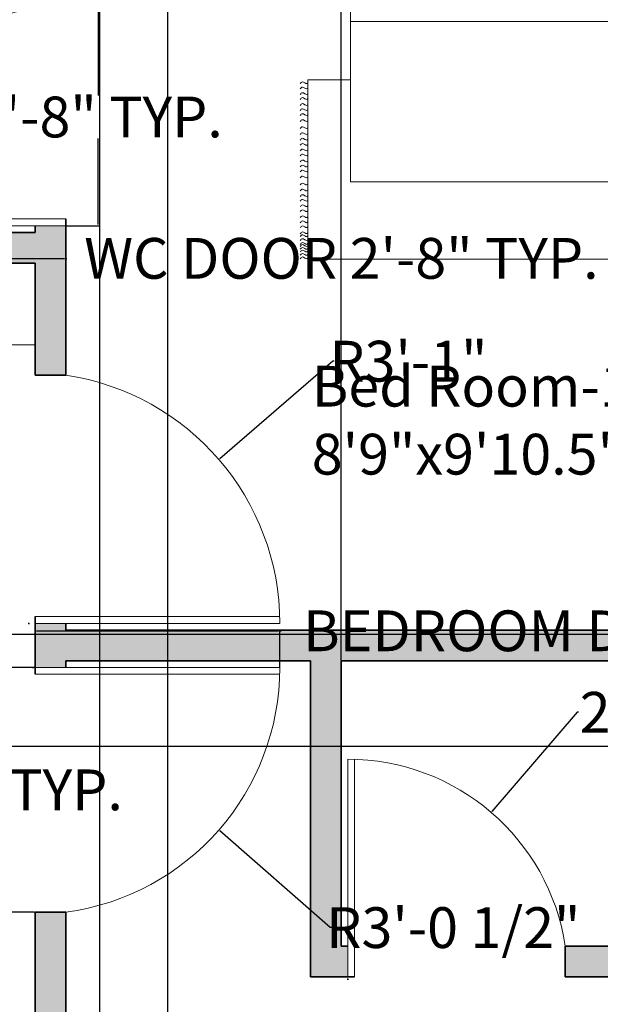
# Model space of a CAD drawing. Units: inches. Extents: x 335 to 688, y 1043 to 1486.
# Tile 5 of 7: x 510 to 596, y 1258 to 1403. Entities that reach past the tile are written whole.
import ezdxf

# ---------------------------------------------------------------- set-up
doc = ezdxf.new("R2010")
doc.units = ezdxf.units.IN
doc.header["$MEASUREMENT"] = 0
for name, color, linetype, lineweight in [('A-ANNO-DIMS', 2, 'Continuous', 18), ('A-AREA-IDEN', 7, 'Continuous', 18), ('A-DOOR', 4, 'Continuous', 18), ('A-FLOR-CASE', 8, 'Continuous', 18), ('A-FURN', 8, 'Continuous', 18), ('A-WALL', 7, 'Continuous', 35), ('A-WALL-PATT', 252, 'Continuous', 13)]:
    doc.layers.add(name, color=color, linetype=linetype, lineweight=lineweight)
doc.styles.get("Standard").update_dxf_attribs({"font": 'arial.ttf'})
doc.dimstyles.get("Standard").update_dxf_attribs({"dimtxt": 6, "dimasz": 0.18, "dimexe": 0.18, "dimexo": 0.0625, "dimgap": 0.09, "dimtad": 0, "dimtih": 1, "dimtoh": 1, "dimdec": 1, "dimzin": 0, "dimdsep": 46, "dimlunit": 3, "dimtxsty": 'Standard', "dimcen": 0.09, "dimadec": 0, "dimazin": 0, "dimtfac": 1, "dimtdec": 1, "dimtofl": 0, "dimtmove": 0, "dimatfit": 3, "dimfxl": 1, "dimtolj": 1, "dimtzin": 0, "dimarcsym": 0})

# ---------------------------------------------------------------- blocks, each defined once
blk = doc.blocks.new('BED-DOUBLE-WITH-NIGHTSTANDS')
for p, q in [((56.59, 58.08), (56.59, 68.14)), ((0, 64.35), (26.37, 64.35)), ((0, 1.12), (0, 64.35)), ((26.37, 64.35), (26.37, 58.06)), ((61.62, 63.11), (51.56, 63.11)), ((34.96, 10.66), (34.96, 58.08)), ((52, 19.27), (52, 58.08)), ((52.82, 19.32), (52.82, 58.08)), ((52.82, 19.32), (46.47, 10.71)), ((52.82, 19.27), (46.47, 19.27)), ((46.47, 19.27), (46.47, 10.71)), ((26.37, 10.66), (26.37, 1.12)), ((56.69, 0.03), (56.69, 10.09)), ((61.72, 5.06), (51.66, 5.06)), ((26.37, 1.12), (0, 1.12))]:
    blk.add_line(p, q)
for points in [[(50.39, 68.71), (50.5, 58.08), (62.68, 58.08), (62.58, 68.71)], [(62.68, 10.66), (11.37, 10.66), (11.37, 58.08), (62.68, 58.08)], [(59.98, 38.83), (52.82, 38.83), (52.82, 52.73), (59.98, 52.73)], [(59.98, 19.27), (52.82, 19.27), (52.82, 33.16), (59.98, 33.16)], [(50.5, 10.66), (50.6, 0.03), (62.78, 0.03), (62.68, 10.66)]]:
    blk.add_lwpolyline(points, close=True)
for centre in [(56.59, 63.11), (56.69, 5.06)]:
    blk.add_circle(centre, 3.92)
for points, knots in [([(0.07, 65.48), (0.19, 65.39), (0.43, 65.19), (0.19, 64.85), (0.02, 64.57), (0.13, 64.42), (0.18, 64.35)], [0, 0, 0, 0, 0.400747, 0.791423, 1.067667, 1.29709, 1.29709, 1.29709, 1.29709]), ([(0.57, 65.48), (0.7, 65.39), (0.94, 65.19), (0.7, 64.85), (0.52, 64.57), (0.63, 64.42), (0.68, 64.35)], [0, 0, 0, 0, 0.400747, 0.791423, 1.067667, 1.29709, 1.29709, 1.29709, 1.29709]), ([(1.06, 65.48), (1.18, 65.39), (1.42, 65.19), (1.18, 64.85), (1.01, 64.57), (1.11, 64.42), (1.16, 64.35)], [0, 0, 0, 0, 0.400747, 0.791423, 1.067667, 1.29709, 1.29709, 1.29709, 1.29709]), ([(1.46, 65.48), (1.58, 65.39), (1.82, 65.19), (1.58, 64.85), (1.41, 64.57), (1.51, 64.42), (1.56, 64.35)], [0, 0, 0, 0, 0.400747, 0.791423, 1.067667, 1.29709, 1.29709, 1.29709, 1.29709]), ([(1.88, 65.48), (2, 65.39), (2.24, 65.19), (2, 64.85), (1.82, 64.57), (1.93, 64.42), (1.98, 64.35)], [0, 0, 0, 0, 0.400747, 0.791423, 1.067667, 1.29709, 1.29709, 1.29709, 1.29709]), ([(2.18, 65.48), (2.31, 65.39), (2.55, 65.19), (2.31, 64.85), (2.13, 64.57), (2.24, 64.42), (2.29, 64.35)], [0, 0, 0, 0, 0.400747, 0.791423, 1.067667, 1.29709, 1.29709, 1.29709, 1.29709]), ([(2.76, 65.48), (2.88, 65.39), (3.12, 65.19), (2.88, 64.85), (2.71, 64.57), (2.81, 64.42), (2.86, 64.35)], [0, 0, 0, 0, 0.400747, 0.791423, 1.067667, 1.29709, 1.29709, 1.29709, 1.29709]), ([(3.33, 65.48), (3.45, 65.39), (3.7, 65.19), (3.44, 64.85), (3.27, 64.57), (3.38, 64.42), (3.43, 64.35)], [0, 0, 0, 0, 0.407265, 0.802015, 1.07826, 1.307683, 1.307683, 1.307683, 1.307683]), ([(3.75, 65.48), (3.88, 65.39), (4.12, 65.19), (3.88, 64.85), (3.7, 64.57), (3.81, 64.42), (3.86, 64.35)], [0, 0, 0, 0, 0.400747, 0.791423, 1.067667, 1.29709, 1.29709, 1.29709, 1.29709]), ([(4.64, 65.48), (4.76, 65.39), (5, 65.19), (4.76, 64.85), (4.59, 64.57), (4.69, 64.42), (4.74, 64.35)], [0, 0, 0, 0, 0.400747, 0.791423, 1.067667, 1.29709, 1.29709, 1.29709, 1.29709]), ([(5.36, 65.48), (5.49, 65.39), (5.73, 65.19), (5.49, 64.85), (5.31, 64.57), (5.42, 64.42), (5.47, 64.35)], [0, 0, 0, 0, 0.400747, 0.791423, 1.067667, 1.29709, 1.29709, 1.29709, 1.29709]), ([(6.12, 65.48), (6.24, 65.39), (6.48, 65.19), (6.24, 64.85), (6.07, 64.57), (6.17, 64.42), (6.22, 64.35)], [0, 0, 0, 0, 0.400747, 0.791423, 1.067667, 1.29709, 1.29709, 1.29709, 1.29709]), ([(7, 65.48), (7.12, 65.39), (7.36, 65.19), (7.12, 64.85), (6.95, 64.57), (7.05, 64.42), (7.1, 64.35)], [0, 0, 0, 0, 0.400747, 0.791423, 1.067667, 1.29709, 1.29709, 1.29709, 1.29709]), ([(7.73, 65.48), (7.85, 65.39), (8.09, 65.19), (7.85, 64.85), (7.68, 64.57), (7.78, 64.42), (7.83, 64.35)], [0, 0, 0, 0, 0.400747, 0.791423, 1.067667, 1.29709, 1.29709, 1.29709, 1.29709]), ([(8.54, 65.48), (8.66, 65.39), (8.9, 65.19), (8.66, 64.85), (8.49, 64.57), (8.6, 64.42), (8.65, 64.35)], [0, 0, 0, 0, 0.400747, 0.791423, 1.067667, 1.29709, 1.29709, 1.29709, 1.29709]), ([(9.23, 65.48), (9.35, 65.39), (9.59, 65.19), (9.35, 64.85), (9.18, 64.57), (9.29, 64.42), (9.34, 64.35)], [0, 0, 0, 0, 0.400747, 0.791423, 1.067667, 1.29709, 1.29709, 1.29709, 1.29709]), ([(10.05, 65.48), (10.17, 65.39), (10.41, 65.19), (10.17, 64.85), (10, 64.57), (10.1, 64.42), (10.15, 64.35)], [0, 0, 0, 0, 0.400747, 0.791423, 1.067667, 1.29709, 1.29709, 1.29709, 1.29709]), ([(10.93, 65.48), (11.05, 65.39), (11.29, 65.19), (11.05, 64.85), (10.88, 64.57), (10.99, 64.42), (11.03, 64.35)], [0, 0, 0, 0, 0.400747, 0.791423, 1.067667, 1.29709, 1.29709, 1.29709, 1.29709]), ([(11.97, 65.48), (12.09, 65.39), (12.33, 65.19), (12.09, 64.85), (11.92, 64.57), (12.02, 64.42), (12.07, 64.35)], [0, 0, 0, 0, 0.400747, 0.791423, 1.067667, 1.29709, 1.29709, 1.29709, 1.29709]), ([(12.85, 65.48), (12.97, 65.39), (13.21, 65.19), (12.97, 64.85), (12.8, 64.57), (12.9, 64.42), (12.95, 64.35)], [0, 0, 0, 0, 0.400747, 0.791423, 1.067667, 1.29709, 1.29709, 1.29709, 1.29709]), ([(13.58, 65.48), (13.7, 65.39), (13.94, 65.19), (13.7, 64.85), (13.53, 64.57), (13.63, 64.42), (13.68, 64.35)], [0, 0, 0, 0, 0.400747, 0.791423, 1.067667, 1.29709, 1.29709, 1.29709, 1.29709]), ([(14.33, 65.48), (14.45, 65.39), (14.69, 65.19), (14.45, 64.85), (14.28, 64.57), (14.38, 64.42), (14.43, 64.35)], [0, 0, 0, 0, 0.400747, 0.791423, 1.067667, 1.29709, 1.29709, 1.29709, 1.29709]), ([(15.21, 65.48), (15.33, 65.39), (15.57, 65.19), (15.33, 64.85), (15.16, 64.57), (15.27, 64.42), (15.32, 64.35)], [0, 0, 0, 0, 0.400747, 0.791423, 1.067667, 1.29709, 1.29709, 1.29709, 1.29709]), ([(15.94, 65.48), (16.06, 65.39), (16.3, 65.19), (16.06, 64.85), (15.89, 64.57), (16, 64.42), (16.04, 64.35)], [0, 0, 0, 0, 0.400747, 0.791423, 1.067667, 1.29709, 1.29709, 1.29709, 1.29709]), ([(16.76, 65.48), (16.88, 65.39), (17.12, 65.19), (16.88, 64.85), (16.7, 64.57), (16.81, 64.42), (16.86, 64.35)], [0, 0, 0, 0, 0.400747, 0.791423, 1.067667, 1.29709, 1.29709, 1.29709, 1.29709]), ([(17.53, 65.48), (17.65, 65.39), (17.89, 65.19), (17.65, 64.85), (17.48, 64.57), (17.59, 64.42), (17.64, 64.35)], [0, 0, 0, 0, 0.400747, 0.791423, 1.067667, 1.29709, 1.29709, 1.29709, 1.29709]), ([(18.35, 65.48), (18.47, 65.39), (18.71, 65.19), (18.47, 64.85), (18.3, 64.57), (18.4, 64.42), (18.45, 64.35)], [0, 0, 0, 0, 0.400747, 0.791423, 1.067667, 1.29709, 1.29709, 1.29709, 1.29709]), ([(19.23, 65.48), (19.35, 65.39), (19.59, 65.19), (19.35, 64.85), (19.18, 64.57), (19.29, 64.42), (19.33, 64.35)], [0, 0, 0, 0, 0.400747, 0.791423, 1.067667, 1.29709, 1.29709, 1.29709, 1.29709]), ([(20.27, 65.48), (20.39, 65.39), (20.63, 65.19), (20.39, 64.85), (20.22, 64.57), (20.32, 64.42), (20.37, 64.35)], [0, 0, 0, 0, 0.400747, 0.791423, 1.067667, 1.29709, 1.29709, 1.29709, 1.29709]), ([(21.15, 65.48), (21.27, 65.39), (21.51, 65.19), (21.27, 64.85), (21.1, 64.57), (21.21, 64.42), (21.25, 64.35)], [0, 0, 0, 0, 0.400747, 0.791423, 1.067667, 1.29709, 1.29709, 1.29709, 1.29709]), ([(21.88, 65.48), (22, 65.39), (22.24, 65.19), (22, 64.85), (21.83, 64.57), (21.93, 64.42), (21.98, 64.35)], [0, 0, 0, 0, 0.400747, 0.791423, 1.067667, 1.29709, 1.29709, 1.29709, 1.29709]), ([(22.63, 65.48), (22.75, 65.39), (22.99, 65.19), (22.75, 64.85), (22.58, 64.57), (22.69, 64.42), (22.73, 64.35)], [0, 0, 0, 0, 0.400747, 0.791423, 1.067667, 1.29709, 1.29709, 1.29709, 1.29709]), ([(23.51, 65.48), (23.63, 65.39), (23.87, 65.19), (23.63, 64.85), (23.46, 64.57), (23.57, 64.42), (23.62, 64.35)], [0, 0, 0, 0, 0.400747, 0.791423, 1.067667, 1.29709, 1.29709, 1.29709, 1.29709]), ([(24.24, 65.48), (24.36, 65.39), (24.6, 65.19), (24.36, 64.85), (24.19, 64.57), (24.3, 64.42), (24.34, 64.35)], [0, 0, 0, 0, 0.400747, 0.791423, 1.067667, 1.29709, 1.29709, 1.29709, 1.29709]), ([(25.06, 65.48), (25.18, 65.39), (25.42, 65.19), (25.18, 64.85), (25.01, 64.57), (25.11, 64.42), (25.16, 64.35)], [0, 0, 0, 0, 0.400747, 0.791423, 1.067667, 1.29709, 1.29709, 1.29709, 1.29709]), ([(25.84, 65.48), (25.96, 65.39), (26.2, 65.19), (25.96, 64.85), (25.78, 64.57), (25.89, 64.42), (25.94, 64.35)], [0, 0, 0, 0, 0.400747, 0.791423, 1.067667, 1.29709, 1.29709, 1.29709, 1.29709]), ([(0.07, 0), (0.19, 0.1), (0.43, 0.29), (0.19, 0.63), (0.02, 0.91), (0.13, 1.06), (0.18, 1.13)], [0, 0, 0, 0, 0.400747, 0.791423, 1.067667, 1.29709, 1.29709, 1.29709, 1.29709]), ([(0.55, 0), (0.67, 0.1), (0.91, 0.29), (0.67, 0.63), (0.49, 0.91), (0.6, 1.06), (0.65, 1.13)], [0, 0, 0, 0, 0.400747, 0.791423, 1.067667, 1.29709, 1.29709, 1.29709, 1.29709]), ([(1.03, 0), (1.15, 0.1), (1.39, 0.29), (1.15, 0.63), (0.98, 0.91), (1.09, 1.06), (1.13, 1.13)], [0, 0, 0, 0, 0.400747, 0.791423, 1.067667, 1.29709, 1.29709, 1.29709, 1.29709]), ([(1.43, 0), (1.55, 0.1), (1.79, 0.29), (1.55, 0.63), (1.38, 0.91), (1.48, 1.06), (1.53, 1.13)], [0, 0, 0, 0, 0.400747, 0.791423, 1.067667, 1.29709, 1.29709, 1.29709, 1.29709]), ([(1.85, 0), (1.97, 0.1), (2.21, 0.29), (1.97, 0.63), (1.8, 0.91), (1.9, 1.05), (1.94, 1.12)], [0, 0, 0, 0, 0.400747, 0.791423, 1.067667, 1.283686, 1.283686, 1.283686, 1.283686]), ([(2.16, 0), (2.28, 0.1), (2.52, 0.29), (2.28, 0.63), (2.11, 0.91), (2.21, 1.05), (2.25, 1.12)], [0, 0, 0, 0, 0.400747, 0.791423, 1.067667, 1.283686, 1.283686, 1.283686, 1.283686]), ([(2.73, 0), (2.85, 0.1), (3.09, 0.29), (2.85, 0.63), (2.68, 0.91), (2.78, 1.05), (2.82, 1.12)], [0, 0, 0, 0, 0.400747, 0.791423, 1.067667, 1.283686, 1.283686, 1.283686, 1.283686]), ([(3.33, 0), (3.45, 0.1), (3.69, 0.29), (3.45, 0.63), (3.28, 0.91), (3.38, 1.05), (3.42, 1.12)], [0, 0, 0, 0, 0.402903, 0.794912, 1.071156, 1.287177, 1.287177, 1.287177, 1.287177]), ([(3.75, 0), (3.88, 0.1), (4.12, 0.29), (3.88, 0.63), (3.7, 0.91), (3.81, 1.05), (3.85, 1.12)], [0, 0, 0, 0, 0.400747, 0.791423, 1.067667, 1.283686, 1.283686, 1.283686, 1.283686]), ([(4.64, 0), (4.76, 0.1), (5, 0.29), (4.76, 0.63), (4.59, 0.91), (4.69, 1.05), (4.73, 1.12)], [0, 0, 0, 0, 0.400747, 0.791423, 1.067667, 1.283686, 1.283686, 1.283686, 1.283686]), ([(5.36, 0), (5.49, 0.1), (5.73, 0.29), (5.49, 0.63), (5.31, 0.91), (5.42, 1.06), (5.47, 1.13)], [0, 0, 0, 0, 0.400747, 0.791423, 1.067667, 1.29709, 1.29709, 1.29709, 1.29709]), ([(6.12, 0), (6.24, 0.1), (6.48, 0.29), (6.24, 0.63), (6.07, 0.91), (6.17, 1.06), (6.22, 1.13)], [0, 0, 0, 0, 0.400747, 0.791423, 1.067667, 1.29709, 1.29709, 1.29709, 1.29709]), ([(7, 0), (7.12, 0.1), (7.36, 0.29), (7.12, 0.63), (6.95, 0.91), (7.05, 1.06), (7.1, 1.13)], [0, 0, 0, 0, 0.400747, 0.791423, 1.067667, 1.29709, 1.29709, 1.29709, 1.29709]), ([(7.73, 0), (7.85, 0.1), (8.09, 0.29), (7.85, 0.63), (7.68, 0.91), (7.78, 1.06), (7.83, 1.13)], [0, 0, 0, 0, 0.400747, 0.791423, 1.067667, 1.29709, 1.29709, 1.29709, 1.29709]), ([(8.54, 0), (8.66, 0.1), (8.9, 0.29), (8.66, 0.63), (8.49, 0.91), (8.6, 1.06), (8.65, 1.13)], [0, 0, 0, 0, 0.400747, 0.791423, 1.067667, 1.29709, 1.29709, 1.29709, 1.29709]), ([(9.23, 0), (9.35, 0.1), (9.59, 0.29), (9.35, 0.63), (9.18, 0.91), (9.29, 1.06), (9.34, 1.13)], [0, 0, 0, 0, 0.400747, 0.791423, 1.067667, 1.29709, 1.29709, 1.29709, 1.29709]), ([(10.05, 0), (10.17, 0.1), (10.41, 0.29), (10.17, 0.63), (10, 0.91), (10.1, 1.06), (10.15, 1.13)], [0, 0, 0, 0, 0.400747, 0.791423, 1.067667, 1.29709, 1.29709, 1.29709, 1.29709]), ([(10.93, 0), (11.05, 0.1), (11.29, 0.29), (11.05, 0.63), (10.88, 0.91), (10.99, 1.06), (11.03, 1.13)], [0, 0, 0, 0, 0.400747, 0.791423, 1.067667, 1.29709, 1.29709, 1.29709, 1.29709]), ([(11.97, 0), (12.09, 0.1), (12.33, 0.29), (12.09, 0.63), (11.92, 0.91), (12.02, 1.06), (12.07, 1.13)], [0, 0, 0, 0, 0.400747, 0.791423, 1.067667, 1.29709, 1.29709, 1.29709, 1.29709]), ([(12.85, 0), (12.97, 0.1), (13.21, 0.29), (12.97, 0.63), (12.8, 0.91), (12.9, 1.06), (12.95, 1.13)], [0, 0, 0, 0, 0.400747, 0.791423, 1.067667, 1.29709, 1.29709, 1.29709, 1.29709]), ([(13.58, 0), (13.7, 0.1), (13.94, 0.29), (13.7, 0.63), (13.53, 0.91), (13.63, 1.06), (13.68, 1.13)], [0, 0, 0, 0, 0.400747, 0.791423, 1.067667, 1.29709, 1.29709, 1.29709, 1.29709]), ([(14.33, 0), (14.45, 0.1), (14.69, 0.29), (14.45, 0.63), (14.28, 0.91), (14.38, 1.06), (14.43, 1.13)], [0, 0, 0, 0, 0.400747, 0.791423, 1.067667, 1.29709, 1.29709, 1.29709, 1.29709]), ([(15.21, 0), (15.33, 0.1), (15.57, 0.29), (15.33, 0.63), (15.16, 0.91), (15.27, 1.06), (15.32, 1.13)], [0, 0, 0, 0, 0.400747, 0.791423, 1.067667, 1.29709, 1.29709, 1.29709, 1.29709]), ([(15.94, 0), (16.06, 0.1), (16.3, 0.29), (16.06, 0.63), (15.89, 0.91), (16, 1.06), (16.04, 1.13)], [0, 0, 0, 0, 0.400747, 0.791423, 1.067667, 1.29709, 1.29709, 1.29709, 1.29709]), ([(16.76, 0), (16.88, 0.1), (17.12, 0.29), (16.88, 0.63), (16.7, 0.91), (16.81, 1.06), (16.86, 1.13)], [0, 0, 0, 0, 0.400747, 0.791423, 1.067667, 1.29709, 1.29709, 1.29709, 1.29709]), ([(17.53, 0), (17.65, 0.1), (17.89, 0.29), (17.65, 0.63), (17.48, 0.91), (17.59, 1.06), (17.64, 1.13)], [0, 0, 0, 0, 0.400747, 0.791423, 1.067667, 1.29709, 1.29709, 1.29709, 1.29709]), ([(18.35, 0), (18.47, 0.1), (18.71, 0.29), (18.47, 0.63), (18.3, 0.91), (18.4, 1.06), (18.45, 1.13)], [0, 0, 0, 0, 0.400747, 0.791423, 1.067667, 1.29709, 1.29709, 1.29709, 1.29709]), ([(19.23, 0), (19.35, 0.1), (19.59, 0.29), (19.35, 0.63), (19.18, 0.91), (19.29, 1.06), (19.33, 1.13)], [0, 0, 0, 0, 0.400747, 0.791423, 1.067667, 1.29709, 1.29709, 1.29709, 1.29709]), ([(20.27, 0), (20.39, 0.1), (20.63, 0.29), (20.39, 0.63), (20.22, 0.91), (20.32, 1.06), (20.37, 1.13)], [0, 0, 0, 0, 0.400747, 0.791423, 1.067667, 1.29709, 1.29709, 1.29709, 1.29709]), ([(21.15, 0), (21.27, 0.1), (21.51, 0.29), (21.27, 0.63), (21.1, 0.91), (21.21, 1.06), (21.25, 1.13)], [0, 0, 0, 0, 0.400747, 0.791423, 1.067667, 1.29709, 1.29709, 1.29709, 1.29709]), ([(21.88, 0), (22, 0.1), (22.24, 0.29), (22, 0.63), (21.83, 0.91), (21.93, 1.06), (21.98, 1.13)], [0, 0, 0, 0, 0.400747, 0.791423, 1.067667, 1.29709, 1.29709, 1.29709, 1.29709]), ([(22.63, 0), (22.75, 0.1), (22.99, 0.29), (22.75, 0.63), (22.58, 0.91), (22.69, 1.06), (22.73, 1.13)], [0, 0, 0, 0, 0.400747, 0.791423, 1.067667, 1.29709, 1.29709, 1.29709, 1.29709]), ([(23.51, 0), (23.63, 0.1), (23.87, 0.29), (23.63, 0.63), (23.46, 0.91), (23.57, 1.06), (23.62, 1.13)], [0, 0, 0, 0, 0.400747, 0.791423, 1.067667, 1.29709, 1.29709, 1.29709, 1.29709]), ([(24.24, 0), (24.36, 0.1), (24.6, 0.29), (24.36, 0.63), (24.19, 0.91), (24.3, 1.06), (24.34, 1.13)], [0, 0, 0, 0, 0.400747, 0.791423, 1.067667, 1.29709, 1.29709, 1.29709, 1.29709]), ([(25.06, 0), (25.18, 0.1), (25.42, 0.29), (25.18, 0.63), (25.01, 0.91), (25.11, 1.06), (25.16, 1.13)], [0, 0, 0, 0, 0.400747, 0.791423, 1.067667, 1.29709, 1.29709, 1.29709, 1.29709]), ([(25.84, 0), (25.96, 0.1), (26.2, 0.29), (25.96, 0.63), (25.78, 0.91), (25.89, 1.06), (25.94, 1.13)], [0, 0, 0, 0, 0.400747, 0.791423, 1.067667, 1.29709, 1.29709, 1.29709, 1.29709])]:
    blk.add_open_spline(points, degree=3, knots=knots)
blk = doc.blocks.new('DOOR-32IN')
for p, q in [((0, 1), (32, 1)), ((32, 0), (32, 1)), ((32, 0), (0, 0)), ((0, 0), (32, 0))]:
    blk.add_line(p, q)
blk.add_arc((32.37, 0), 32.37, 98.6501, 180)
blk = doc.blocks.new('DOOR-36IN')
for p, q in [((0, 36), (36, 36)), ((36, 35), (0, 35))]:
    blk.add_line(p, q)
blk.add_arc((-0.32, 36), 36.32, 277.6281, 0)
blk = doc.blocks.new('*D29')
at = {"layer": 'A-ANNO-DIMS', "color": 0, "lineweight": -2, "transparency": 16777216}
for p, q in [((485.11, 1372.9), (485.11, 1367.99)), ((517.11, 1372.9), (517.11, 1367.99)), ((485.29, 1368.17), (516.93, 1368.17)), ((517.11, 1368.17), (517.29, 1368.17))]:
    blk.add_line(p, q, dxfattribs=at)
at = {"layer": 'A-ANNO-DIMS', "color": 0, "transparency": 16777216}
for points in [[(485.29, 1368.2), (485.29, 1368.14), (485.11, 1368.17)], [(516.93, 1368.2), (516.93, 1368.14), (517.11, 1368.17)]]:
    blk.add_solid(points, dxfattribs=at)
at = {"layer": 'Defpoints', "color": 0, "transparency": 16777216}
for p in [(485.11, 1372.97), (517.11, 1372.97), (517.11, 1368.17)]:
    blk.add_point(p, dxfattribs=at)
at = {"layer": 'A-ANNO-DIMS', "color": 0, "transparency": 16777216, "insert": (557.67, 1368.17), "char_height": 6, "attachment_point": 5}
blk.add_mtext('\\A1;WC DOOR 2\'-8" TYP.', dxfattribs=at)
blk = doc.blocks.new('*D30')
at = {"layer": 'A-ANNO-DIMS', "color": 0, "lineweight": -2, "transparency": 16777216}
for p, q in [((517.17, 1404.97), (522.09, 1404.97)), ((521.91, 1404.79), (521.91, 1392.12)), ((521.91, 1373.15), (521.91, 1385.81)), ((517.17, 1372.97), (522.09, 1372.97))]:
    blk.add_line(p, q, dxfattribs=at)
at = {"layer": 'A-ANNO-DIMS', "color": 0, "transparency": 16777216}
for points in [[(521.88, 1404.79), (521.94, 1404.79), (521.91, 1404.97)], [(521.88, 1373.15), (521.94, 1373.15), (521.91, 1372.97)]]:
    blk.add_solid(points, dxfattribs=at)
at = {"layer": 'Defpoints', "color": 0, "transparency": 16777216}
for p in [(517.11, 1404.97), (521.91, 1404.97), (517.11, 1372.97)]:
    blk.add_point(p, dxfattribs=at)
at = {"layer": 'A-ANNO-DIMS', "color": 0, "transparency": 16777216, "insert": (521.91, 1388.97), "char_height": 6, "attachment_point": 5}
blk.add_mtext('\\A1;2\'-8" TYP.', dxfattribs=at)
blk = doc.blocks.new('*D31')
at = {"layer": 'A-ANNO-DIMS', "color": 0, "lineweight": -2, "transparency": 16777216}
for p, q in [((512.61, 1308.03), (512.61, 1313.55)), ((512.79, 1313.37), (548.43, 1313.37)), ((548.61, 1308.03), (548.61, 1313.55)), ((548.61, 1313.37), (548.79, 1313.37))]:
    blk.add_line(p, q, dxfattribs=at)
at = {"layer": 'A-ANNO-DIMS', "color": 0, "transparency": 16777216}
for points in [[(512.79, 1313.4), (512.79, 1313.34), (512.61, 1313.37)], [(548.43, 1313.4), (548.43, 1313.34), (548.61, 1313.37)]]:
    blk.add_solid(points, dxfattribs=at)
at = {"layer": 'Defpoints', "color": 0, "transparency": 16777216}
for p in [(548.61, 1313.37), (512.61, 1307.97), (548.61, 1307.97)]:
    blk.add_point(p, dxfattribs=at)
at = {"layer": 'A-ANNO-DIMS', "color": 0, "transparency": 16777216, "insert": (603.59, 1313.37), "char_height": 6, "attachment_point": 5}
blk.add_mtext('\\A1;BEDROOM DOOR 3\'-0" TYP.', dxfattribs=at)
blk = doc.blocks.new('*D32')
at = {"layer": 'A-ANNO-DIMS', "color": 0, "lineweight": -2, "transparency": 16777216}
for p, q in [((512.54, 1307.97), (507.03, 1307.97)), ((507.21, 1307.79), (507.21, 1293.12)), ((507.21, 1272.15), (507.21, 1286.81)), ((512.54, 1271.97), (507.03, 1271.97))]:
    blk.add_line(p, q, dxfattribs=at)
at = {"layer": 'A-ANNO-DIMS', "color": 0, "transparency": 16777216}
for points in [[(507.18, 1307.79), (507.24, 1307.79), (507.21, 1307.97)], [(507.18, 1272.15), (507.24, 1272.15), (507.21, 1271.97)]]:
    blk.add_solid(points, dxfattribs=at)
at = {"layer": 'Defpoints', "color": 0, "transparency": 16777216}
for p in [(507.21, 1307.97), (512.61, 1307.97), (512.61, 1271.97)]:
    blk.add_point(p, dxfattribs=at)
at = {"layer": 'A-ANNO-DIMS', "color": 0, "transparency": 16777216, "insert": (507.21, 1289.97), "char_height": 6, "attachment_point": 5}
blk.add_mtext('\\A1;3\'-0" TYP.', dxfattribs=at)
blk = doc.blocks.new('*D41')
at = {"layer": 'A-ANNO-DIMS', "color": 0, "lineweight": -2, "transparency": 16777216}
for p, q in [((430.31, 1312.88), (650.79, 1312.88)), ((650.61, 1312.7), (650.61, 1307.84)), ((650.61, 1296.6), (650.61, 1301.46)), ((430.31, 1296.42), (650.79, 1296.42))]:
    blk.add_line(p, q, dxfattribs=at)
at = {"layer": 'A-ANNO-DIMS', "color": 0, "transparency": 16777216}
for points in [[(650.58, 1312.7), (650.64, 1312.7), (650.61, 1312.88)], [(650.58, 1296.6), (650.64, 1296.6), (650.61, 1296.42)]]:
    blk.add_solid(points, dxfattribs=at)
at = {"layer": 'Defpoints', "color": 0, "transparency": 16777216}
for p in [(430.25, 1312.88), (650.61, 1312.88), (430.25, 1296.42)]:
    blk.add_point(p, dxfattribs=at)
at = {"layer": 'A-ANNO-DIMS', "color": 0, "transparency": 16777216, "insert": (650.61, 1304.65), "char_height": 6, "attachment_point": 5}
blk.add_mtext('\\A1;1\'-4 1/2"', dxfattribs=at)
blk = doc.blocks.new('*D42')
at = {"layer": 'A-ANNO-DIMS', "color": 0, "lineweight": -2, "transparency": 16777216}
for p, q in [((557.61, 1309.03), (557.61, 1460.65)), ((557.79, 1460.47), (574.8, 1460.47)), ((621.93, 1460.47), (604.91, 1460.47)), ((622.11, 1309.03), (622.11, 1460.65))]:
    blk.add_line(p, q, dxfattribs=at)
at = {"layer": 'A-ANNO-DIMS', "color": 0, "transparency": 16777216}
for points in [[(557.79, 1460.5), (557.79, 1460.44), (557.61, 1460.47)], [(621.93, 1460.5), (621.93, 1460.44), (622.11, 1460.47)]]:
    blk.add_solid(points, dxfattribs=at)
at = {"layer": 'Defpoints', "color": 0, "transparency": 16777216}
for p in [(622.11, 1460.47), (557.61, 1308.97), (622.11, 1308.97)]:
    blk.add_point(p, dxfattribs=at)
at = {"layer": 'A-ANNO-DIMS', "color": 0, "transparency": 16777216, "insert": (589.86, 1460.47), "char_height": 6, "attachment_point": 5}
blk.add_mtext('\\A1;5\'-4 1/2"', dxfattribs=at)
blk = doc.blocks.new('*D57')
at = {"layer": 'A-ANNO-DIMS', "color": 0, "lineweight": -2, "transparency": 16777216}
for p, q in [((522.11, 1090.03), (522.11, 1460.65)), ((522.29, 1460.47), (531.93, 1460.47)), ((532.11, 1090.03), (532.11, 1460.65)), ((532.11, 1460.47), (532.29, 1460.47))]:
    blk.add_line(p, q, dxfattribs=at)
at = {"layer": 'A-ANNO-DIMS', "color": 0, "transparency": 16777216}
for points in [[(522.29, 1460.5), (522.29, 1460.44), (522.11, 1460.47)], [(531.93, 1460.5), (531.93, 1460.44), (532.11, 1460.47)]]:
    blk.add_solid(points, dxfattribs=at)
at = {"layer": 'Defpoints', "color": 0, "transparency": 16777216}
for p in [(532.11, 1460.47), (522.11, 1089.97), (532.11, 1089.97)]:
    blk.add_point(p, dxfattribs=at)
at = {"layer": 'A-ANNO-DIMS', "color": 0, "transparency": 16777216, "insert": (542.68, 1460.47), "char_height": 6, "attachment_point": 5}
blk.add_mtext('\\A1;0\'-10"', dxfattribs=at)
blk = doc.blocks.new('*D64')
at = {"layer": 'A-ANNO-DIMS', "color": 0, "lineweight": -2, "transparency": 16777216}
for p, q in [((556.4, 1353.04), (539.78, 1338.69)), ((556.58, 1353.04), (556.4, 1353.04)), ((511.62, 1314.47), (511.8, 1314.47)), ((511.71, 1314.38), (511.71, 1314.56))]:
    blk.add_line(p, q, dxfattribs=at)
at = {"layer": 'A-ANNO-DIMS', "color": 0, "transparency": 16777216}
blk.add_solid([(539.76, 1338.71), (539.8, 1338.67), (539.64, 1338.57)], dxfattribs=at)
at = {"layer": 'Defpoints', "color": 0, "transparency": 16777216}
for p in [(539.64, 1338.57), (511.71, 1314.47)]:
    blk.add_point(p, dxfattribs=at)
at = {"layer": 'A-ANNO-DIMS', "color": 0, "transparency": 16777216, "insert": (567.52, 1353.04), "char_height": 6, "attachment_point": 5}
blk.add_mtext('\\A1;R3\'-1"', dxfattribs=at)
blk = doc.blocks.new('*D65')
at = {"layer": 'A-ANNO-DIMS', "color": 0, "lineweight": -2, "transparency": 16777216}
for p, q in [((512.19, 1307.97), (512.37, 1307.97)), ((512.28, 1307.88), (512.28, 1308.06)), ((556.02, 1269.7), (539.76, 1283.93)), ((556.2, 1269.7), (556.02, 1269.7))]:
    blk.add_line(p, q, dxfattribs=at)
at = {"layer": 'A-ANNO-DIMS', "color": 0, "transparency": 16777216}
blk.add_solid([(539.78, 1283.95), (539.74, 1283.91), (539.62, 1284.05)], dxfattribs=at)
at = {"layer": 'Defpoints', "color": 0, "transparency": 16777216}
for p in [(512.28, 1307.97), (539.62, 1284.05)]:
    blk.add_point(p, dxfattribs=at)
at = {"layer": 'A-ANNO-DIMS', "color": 0, "transparency": 16777216, "insert": (574.13, 1269.7), "char_height": 6, "attachment_point": 5}
blk.add_mtext('\\A1;R3\'-0 1/2"', dxfattribs=at)
blk = doc.blocks.new('*D66')
at = {"layer": 'A-ANNO-DIMS', "color": 0, "lineweight": -2, "transparency": 16777216}
for p, q in [((592.36, 1301.38), (579.82, 1286.78)), ((592.54, 1301.38), (592.36, 1301.38)), ((558.52, 1262.1), (558.7, 1262.1)), ((558.61, 1262.01), (558.61, 1262.19))]:
    blk.add_line(p, q, dxfattribs=at)
at = {"layer": 'A-ANNO-DIMS', "color": 0, "transparency": 16777216}
blk.add_solid([(579.8, 1286.8), (579.84, 1286.76), (579.7, 1286.65)], dxfattribs=at)
at = {"layer": 'Defpoints', "color": 0, "transparency": 16777216}
for p in [(579.7, 1286.65), (558.61, 1262.1)]:
    blk.add_point(p, dxfattribs=at)
at = {"layer": 'A-ANNO-DIMS', "color": 0, "transparency": 16777216, "insert": (616.96, 1301.38), "char_height": 6, "attachment_point": 5}
blk.add_mtext('\\A1;2X R2\'-8 1/2"', dxfattribs=at)

msp = doc.modelspace()

# ---------------------------------------------------------------- hatches: boundary and pattern name
at = {"layer": 'A-WALL-PATT'}
h = msp.add_hatch(color=256, dxfattribs=at)
h.dxf.hatch_style = 1
h.paths.add_polyline_path([(478.71, 1440.97), (391.11, 1440.97), (391.11, 1411.42), (400.11, 1411.42), (400.11, 1431.97), (466.11, 1431.97), (466.11, 1347.97), (466.11, 1343.47), (470.61, 1343.47), (470.61, 1367.47), (512.61, 1367.47), (512.61, 1350.97), (517.11, 1350.97), (517.11, 1372.97), (512.61, 1372.97), (512.61, 1371.97), (470.61, 1371.97), (470.61, 1431.97), (478.71, 1431.97)])
h.paths.add_polyline_path([(631.11, 1440.97), (502.71, 1440.97), (502.71, 1431.97), (512.61, 1431.97), (512.61, 1404.97), (517.11, 1404.97), (517.11, 1431.97), (622.11, 1431.97), (622.11, 1401.6), (631.11, 1401.6)])
h.paths.add_polyline_path([(631.11, 1341.6), (622.11, 1341.6), (622.11, 1313.47), (517.11, 1313.47), (517.11, 1314.47), (512.61, 1314.47), (512.61, 1313.47), (512.61, 1307.97), (517.11, 1307.97), (517.11, 1308.97), (553.11, 1308.97), (553.11, 1262.47), (558.61, 1262.47), (558.61, 1266.97), (557.61, 1266.97), (557.61, 1308.97), (622.11, 1308.97), (622.11, 1297.63), (631.11, 1297.63)])
h.paths.add_polyline_path([(631.11, 1273.63), (622.11, 1273.63), (622.11, 1266.97), (590.61, 1266.97), (590.61, 1262.47), (622.11, 1262.47), (622.11, 1230.86), (631.11, 1230.86)])
h.paths.add_polyline_path([(400.11, 1253.85), (391.11, 1253.85), (391.11, 1132.26), (400.11, 1132.26), (400.11, 1149.97), (411.11, 1149.97), (411.11, 1154.47), (400.11, 1154.47)], flags=17)
h.paths.add_polyline_path([(400.11, 1375.42), (391.11, 1375.42), (391.11, 1313.85), (400.11, 1313.85), (400.11, 1343.47), (428.36, 1343.47), (428.36, 1347.97), (400.11, 1347.97)])
h = msp.add_hatch(color=256, dxfattribs=at)
h.dxf.hatch_style = 1
h.paths.add_polyline_path([(467.19, 1089.97), (464.61, 1089.97), (464.61, 1149.97), (475.61, 1149.97), (475.61, 1154.47), (459.11, 1154.47), (459.11, 1149.97), (460.11, 1149.97), (460.11, 1089.97), (400.11, 1089.97), (400.11, 1108.26), (391.11, 1108.26), (391.11, 1080.97), (467.19, 1080.97)])
h.paths.add_polyline_path([(631.11, 1170.86), (622.11, 1170.86), (622.11, 1154.47), (517.11, 1154.47), (517.11, 1271.97), (512.61, 1271.97), (512.61, 1154.47), (511.61, 1154.47), (511.61, 1149.97), (512.61, 1149.97), (622.11, 1149.97), (622.11, 1089.97), (518.67, 1089.97), (518.67, 1080.97), (631.11, 1080.97)])

# ---------------------------------------------------------------- linework, layer by layer
at = {"layer": 'A-DOOR'}
for p, q in [((512.61, 1315.47), (548.61, 1315.47)), ((512.61, 1314.47), (548.61, 1314.47)), ((548.61, 1307.97), (512.61, 1307.97)), ((512.61, 1307.97), (512.61, 1306.97))]:
    msp.add_line(p, q, dxfattribs=at)
msp.add_arc((511.71, 1314.47), 36.9, 360, 81.5893, dxfattribs=at)
at = {"layer": 'A-FLOR-CASE'}
msp.add_line((470.61, 1355.47), (512.61, 1355.47), dxfattribs=at)
at = {"layer": 'A-WALL'}
for p, q in [((517.11, 1373.97), (517.11, 1350.97)), ((470.61, 1371.97), (512.61, 1371.97)), ((512.61, 1372.97), (512.61, 1371.97)), ((517.11, 1371.97), (517.11, 1372.97)), ((470.61, 1367.47), (512.61, 1367.47)), ((512.61, 1367.47), (512.61, 1350.97)), ((512.61, 1350.97), (517.11, 1350.97)), ((512.61, 1315.47), (512.61, 1306.97)), ((517.11, 1314.47), (517.11, 1313.47)), ((517.11, 1313.47), (622.11, 1313.47)), ((517.11, 1308.97), (553.11, 1308.97)), ((517.11, 1308.97), (517.11, 1307.97)), ((553.11, 1308.97), (553.11, 1262.47)), ((557.61, 1308.97), (557.61, 1266.97)), ((557.61, 1308.97), (622.11, 1308.97)), ((512.61, 1271.97), (517.11, 1271.97)), ((512.61, 1271.97), (512.61, 1154.47)), ((517.11, 1271.97), (517.11, 1154.47)), ((557.61, 1266.97), (558.61, 1266.97)), ((590.61, 1262.47), (590.61, 1266.97)), ((590.61, 1266.97), (622.11, 1266.97)), ((553.11, 1262.47), (559.61, 1262.47)), ((557.61, 1262.47), (558.61, 1262.47)), ((590.61, 1262.47), (622.11, 1262.47))]:
    msp.add_line(p, q, dxfattribs=at)

# ---------------------------------------------------------------- block references
at = {"layer": 'A-DOOR'}
for name, p in [('DOOR-32IN', (485.11, 1372.97)), ('DOOR-36IN', (512.61, 1271.97))]:
    msp.add_blockref(name, p, dxfattribs=at)
at = {"layer": 'A-DOOR', "rotation": 269.9999999999993}
msp.add_blockref('DOOR-32IN', (558.61, 1294.47), dxfattribs=at)
at = {"layer": 'A-FURN', "rotation": 89.99999999999726}
msp.add_blockref('BED-DOUBLE-WITH-NIGHTSTANDS', (617.1, 1368.05), dxfattribs=at)

# ---------------------------------------------------------------- texts
at = {"layer": 'A-AREA-IDEN', "insert": (553.31, 1352.36), "char_height": 6, "attachment_point": 1}
msp.add_mtext_dynamic_manual_height_columns('Bed Room-1\\P8\'9"x9\'10.5"', width=58.328, gutter_width=1, heights=[0], dxfattribs=at)

# ---------------------------------------------------------------- dimensions: what is measured, and where the dimension line sits
at = {"layer": 'A-ANNO-DIMS'}
for base, p1, p2, picture, middle in [((622.11, 1460.47), (557.61, 1308.97), (622.11, 1308.97), '*D42', (589.86, 1460.47)), ((532.11, 1460.47), (522.11, 1089.97), (532.11, 1089.97), '*D57', (542.68, 1460.47))]:
    dim = msp.add_linear_dim(base=base, p1=p1, p2=p2, dimstyle='Standard', override={"dimdec": 1, "dimlfac": 1, "dimrnd": 0, "dimzin": 1, "dimdsep": 46, "dimlunit": 4, "dimfrac": 2}, dxfattribs=at)
    dim.commit()
    dim.dimension.update_dxf_attribs({"geometry": picture, "text_midpoint": middle})
for base, p1, p2, picture, middle in [((521.91, 1404.97), (517.11, 1372.97), (517.11, 1404.97), '*D30', (521.91, 1388.97)), ((507.21, 1307.97), (512.61, 1271.97), (512.61, 1307.97), '*D32', (507.21, 1289.97))]:
    dim = msp.add_linear_dim(base=base, p1=p1, p2=p2, angle=90, text='<> TYP.', dimstyle='Standard', override={"dimdec": 1, "dimlfac": 1, "dimrnd": 0, "dimzin": 1, "dimdsep": 46, "dimlunit": 4, "dimfrac": 2}, dxfattribs=at)
    dim.commit()
    dim.dimension.update_dxf_attribs({"geometry": picture, "text_midpoint": middle})
for base, p1, p2, text, picture, middle in [((517.11, 1368.17), (485.11, 1372.97), (517.11, 1372.97), 'WC DOOR <> TYP.', '*D29', (557.67, 1368.17)), ((548.61, 1313.37), (512.61, 1307.97), (548.61, 1307.97), 'BEDROOM DOOR <> TYP.', '*D31', (603.59, 1313.37))]:
    dim = msp.add_linear_dim(base=base, p1=p1, p2=p2, text=text, dimstyle='Standard', override={"dimdec": 1, "dimlfac": 1, "dimrnd": 0, "dimzin": 1, "dimdsep": 46, "dimlunit": 4, "dimfrac": 2}, dxfattribs=at)
    dim.commit()
    dim.dimension.update_dxf_attribs({"geometry": picture, "text_midpoint": middle})
for center, mpoint, picture, middle in [((511.71, 1314.47), (539.64, 1338.57), '*D64', (567.52, 1353.04)), ((512.28, 1307.97), (539.62, 1284.05), '*D65', (574.13, 1269.7))]:
    dim = msp.add_radius_dim(center=center, mpoint=mpoint, dimstyle='Standard', override={"dimdec": 1, "dimlfac": 1, "dimrnd": 0, "dimzin": 1, "dimdsep": 46, "dimlunit": 4, "dimfrac": 2}, dxfattribs=at)
    dim.commit()
    dim.dimension.update_dxf_attribs({"geometry": picture, "text_midpoint": middle, "dimtype": 164})
dim = msp.add_radius_dim(center=(558.61, 1262.1), mpoint=(579.7, 1286.65), text='2X <>', dimstyle='Standard', override={"dimdec": 1, "dimlfac": 1, "dimrnd": 0, "dimzin": 1, "dimdsep": 46, "dimlunit": 4, "dimfrac": 2}, dxfattribs=at)
dim.commit()
dim.dimension.update_dxf_attribs({"geometry": '*D66', "text_midpoint": (616.96, 1301.38), "dimtype": 164})
dim = msp.add_linear_dim(base=(650.61, 1312.88), p1=(430.25, 1296.42), p2=(430.25, 1312.88), angle=90, dimstyle='Standard', override={"dimdec": 1, "dimlfac": 1, "dimrnd": 0, "dimzin": 1, "dimdsep": 46, "dimlunit": 4, "dimfrac": 2}, dxfattribs=at)
dim.commit()
dim.dimension.update_dxf_attribs({"geometry": '*D41', "text_midpoint": (650.61, 1304.65)})

doc.saveas('drawing.dxf')
